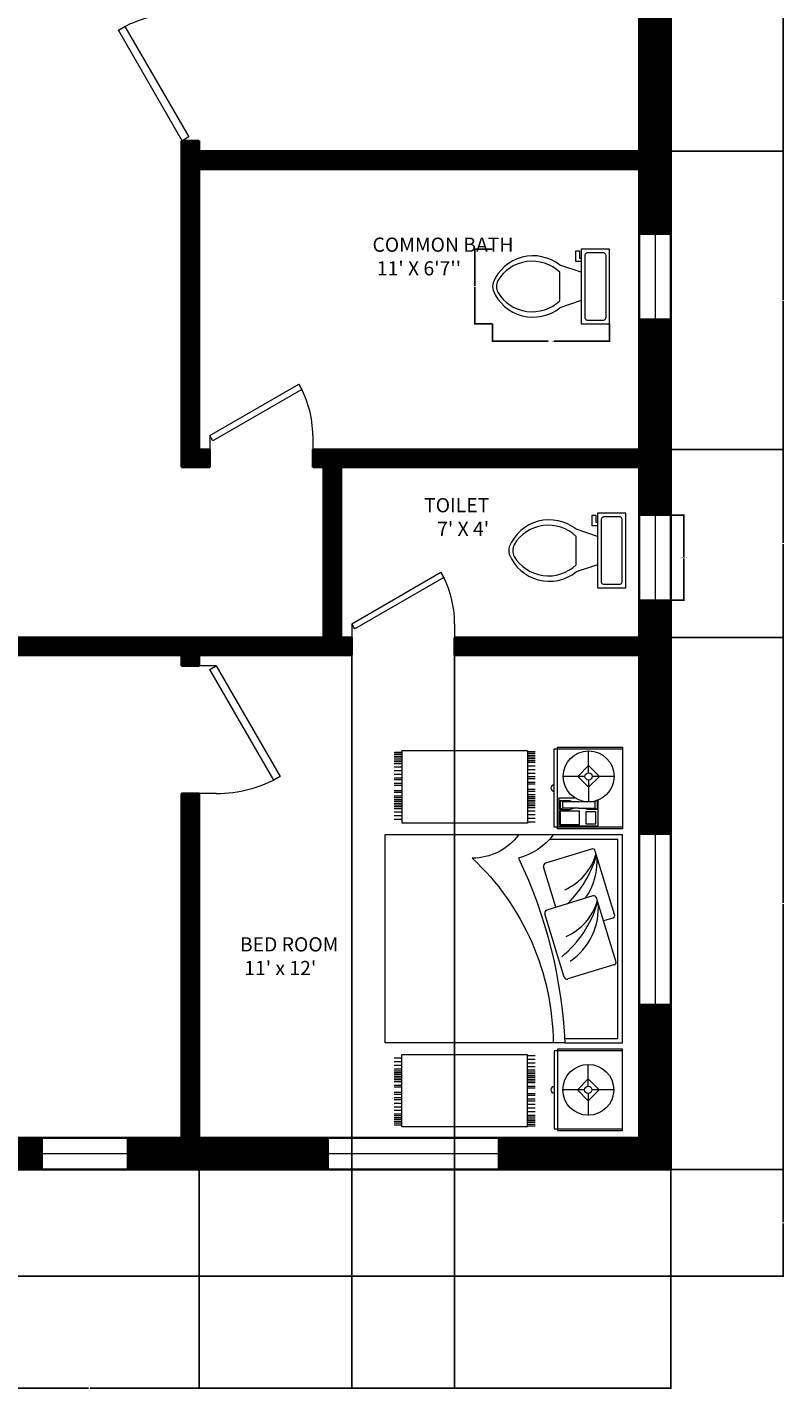
# Model space of a CAD drawing. Units: inches. Extents: x -19 to 404, y -21 to 673.
# Tile 2 of 3: x 191 to 404, y -21 to 363. Entities that reach past the tile are written whole.
import ezdxf

# ---------------------------------------------------------------- set-up
doc = ezdxf.new("R2010")
doc.units = ezdxf.units.IN
doc.header["$MEASUREMENT"] = 0
for name, color, linetype, lineweight in [('A-ANNO-DIMS', 2, 'Continuous', 18), ('A-AREA-IDEN', 7, 'Continuous', 18), ('A-WALL', 7, 'Continuous', 35), ('bathroom', 90, 'Continuous', 18), ('bedroom', 120, 'Continuous', 18), ('doors', 40, 'Continuous', 18), ('window', 30, 'Continuous', 18)]:
    doc.layers.add(name, color=color, linetype=linetype, lineweight=lineweight)
doc.layers.add('A-WALL-PATT', color=244, linetype='Continuous', lineweight=13, true_color=0x991b1e)
doc.styles.get("Standard").update_dxf_attribs({"font": 'arial.ttf'})
doc.dimstyles.get("Standard").update_dxf_attribs({"dimtxt": 0.18, "dimasz": 0.18, "dimexe": 0.18, "dimexo": 0.0625, "dimgap": 0.09, "dimtad": 0, "dimtih": 1, "dimtoh": 1, "dimdec": 4, "dimzin": 0, "dimdsep": 46, "dimtxsty": 'Standard', "dimcen": 0.09, "dimadec": 0, "dimazin": 0, "dimtfac": 1, "dimtdec": 4, "dimtofl": 0, "dimtmove": 0, "dimatfit": 3, "dimfxl": 1, "dimtolj": 1, "dimtzin": 0, "dimarcsym": 0})

# ---------------------------------------------------------------- blocks, each defined once
blk = doc.blocks.new('*U5')
for p, q in [((0, 0), (0, -100)), ((750, 0), (750, -100))]:
    blk.add_line(p, q)
blk.add_lwpolyline([(0, 0), (649.5, 375), (671.4, 337.1), (21.9, -37.9)], close=True)
blk.add_arc((0, 0), 750, 0, 30)
blk = doc.blocks.new('3')
for p, q in [((185.866, 224.677), (185.866, 225.236)), ((185.866, 225.236), (186.566, 225.236)), ((185.88, 224.649), (185.88, 225.236)), ((186.552, 225.236), (186.552, 224.649)), ((186.566, 225.236), (186.566, 224.677)), ((186.62, 225.236), (186.62, 224.64)), ((188.409, 225.236), (186.62, 225.236)), ((188.409, 224.739), (188.409, 225.236)), ((188.463, 225.236), (188.463, 224.677)), ((189.162, 225.236), (188.463, 225.236)), ((188.477, 225.236), (188.477, 224.649)), ((189.148, 224.649), (189.148, 225.236)), ((189.162, 224.677), (189.162, 225.236)), ((186.116, 225.164), (186.116, 224.976)), ((187.303, 225.168), (186.758, 225.001)), ((187.706, 225.179), (187.161, 225.012)), ((187.334, 225.152), (187.359, 225.073)), ((187.737, 225.163), (187.858, 224.766)), ((188.812, 225.162), (188.812, 224.974)), ((186.022, 224.945), (186.116, 225.039)), ((186.116, 225.039), (186.21, 224.945)), ((186.54, 225.027), (186.319, 225.027)), ((186.321, 225.017), (186.401, 225.017)), ((186.333, 224.997), (186.321, 225.017)), ((186.334, 224.858), (186.333, 224.997)), ((186.333, 224.997), (186.389, 224.997)), ((186.401, 225.017), (186.389, 224.997)), ((186.39, 224.858), (186.389, 224.997)), ((186.401, 225.017), (186.401, 224.938)), ((186.541, 224.69), (186.54, 225.027)), ((186.742, 224.97), (186.863, 224.573)), ((187.144, 224.981), (187.266, 224.584)), ((188.812, 225.036), (188.718, 224.942)), ((188.907, 224.942), (188.812, 225.036)), ((186.084, 224.945), (185.896, 224.945)), ((186.116, 224.851), (186.022, 224.945)), ((186.21, 224.945), (186.116, 224.851)), ((186.116, 224.914), (186.116, 224.726)), ((186.147, 224.945), (186.335, 224.945)), ((186.331, 224.905), (186.334, 224.898)), ((186.334, 224.858), (186.334, 224.719)), ((186.401, 224.938), (186.389, 224.898)), ((186.39, 224.858), (186.39, 224.719)), ((188.781, 224.942), (188.593, 224.942)), ((188.718, 224.942), (188.812, 224.848)), ((188.812, 224.848), (188.907, 224.942)), ((188.812, 224.911), (188.812, 224.723)), ((188.844, 224.942), (189.032, 224.942)), ((186.302, 224.83), (186.303, 224.689)), ((186.322, 224.779), (186.334, 224.818)), ((186.323, 224.699), (186.322, 224.779)), ((186.402, 224.779), (186.39, 224.819)), ((186.402, 224.7), (186.402, 224.779)), ((187.842, 224.735), (187.297, 224.568)), ((188.409, 224.739), (188.409, 223.191)), ((186.566, 224.677), (185.866, 224.677)), ((186.552, 224.649), (185.88, 224.649)), ((186.303, 224.689), (186.541, 224.69)), ((186.334, 224.719), (186.323, 224.699)), ((186.323, 224.699), (186.402, 224.7)), ((186.334, 224.719), (186.39, 224.719)), ((186.402, 224.7), (186.39, 224.719)), ((186.62, 224.64), (186.62, 223.191)), ((187.242, 224.663), (186.894, 224.557)), ((188.463, 224.677), (189.162, 224.677)), ((188.477, 224.649), (189.148, 224.649)), ((185.897, 224.42, -0.909), (185.897, 223.338, -0.909)), ((185.897, 224.42, -0.909), (186.517, 224.42, -0.909)), ((185.904, 224.485, -0.909), (185.904, 224.42, -0.909)), ((185.92, 224.485, -0.909), (185.92, 224.42, -0.909)), ((185.92, 224.485, -0.909), (185.92, 224.42, -0.909)), ((185.935, 224.485, -0.909), (185.935, 224.42, -0.909)), ((185.951, 224.485, -0.909), (185.951, 224.42, -0.909)), ((185.966, 224.485, -0.909), (185.966, 224.42, -0.909)), ((185.982, 224.485, -0.909), (185.982, 224.42, -0.909)), ((185.997, 224.485, -0.909), (185.997, 224.42, -0.909)), ((186.028, 224.485, -0.909), (186.028, 224.42, -0.909)), ((186.059, 224.485, -0.909), (186.059, 224.42, -0.909)), ((186.09, 224.485, -0.909), (186.09, 224.42, -0.909)), ((186.09, 224.485, -0.909), (186.09, 224.42, -0.909)), ((186.121, 224.485, -0.909), (186.121, 224.42, -0.909)), ((186.137, 224.485, -0.909), (186.137, 224.42, -0.909)), ((186.168, 224.485, -0.909), (186.168, 224.42, -0.909)), ((186.183, 224.485, -0.909), (186.183, 224.42, -0.909)), ((186.23, 224.485, -0.909), (186.23, 224.42, -0.909)), ((186.245, 224.485, -0.909), (186.245, 224.42, -0.909)), ((186.276, 224.485, -0.909), (186.276, 224.42, -0.909)), ((186.292, 224.485, -0.909), (186.292, 224.42, -0.909)), ((186.307, 224.485, -0.909), (186.307, 224.42, -0.909)), ((186.323, 224.485, -0.909), (186.323, 224.42, -0.909)), ((186.338, 224.485, -0.909), (186.338, 224.42, -0.909)), ((186.354, 224.485, -0.909), (186.354, 224.42, -0.909)), ((186.369, 224.485, -0.909), (186.369, 224.42, -0.909)), ((186.385, 224.485, -0.909), (186.385, 224.42, -0.909)), ((186.416, 224.485, -0.909), (186.416, 224.42, -0.909)), ((186.447, 224.485, -0.909), (186.447, 224.42, -0.909)), ((186.478, 224.485, -0.909), (186.478, 224.42, -0.909)), ((186.509, 224.485, -0.909), (186.509, 224.42, -0.909)), ((186.517, 224.42, -0.909), (186.517, 223.338, -0.909)), ((189.131, 224.42, -0.909), (188.511, 224.42, -0.909)), ((188.511, 224.42, -0.909), (188.511, 223.338, -0.909)), ((188.52, 224.485, -0.909), (188.52, 224.42, -0.909)), ((188.551, 224.485, -0.909), (188.551, 224.42, -0.909)), ((188.582, 224.485, -0.909), (188.582, 224.42, -0.909)), ((188.613, 224.485, -0.909), (188.613, 224.42, -0.909)), ((188.644, 224.485, -0.909), (188.644, 224.42, -0.909)), ((188.66, 224.485, -0.909), (188.66, 224.42, -0.909)), ((188.675, 224.485, -0.909), (188.675, 224.42, -0.909)), ((188.691, 224.485, -0.909), (188.691, 224.42, -0.909)), ((188.706, 224.485, -0.909), (188.706, 224.42, -0.909)), ((188.722, 224.485, -0.909), (188.722, 224.42, -0.909)), ((188.737, 224.485, -0.909), (188.737, 224.42, -0.909)), ((188.753, 224.485, -0.909), (188.753, 224.42, -0.909)), ((188.784, 224.485, -0.909), (188.784, 224.42, -0.909)), ((188.799, 224.485, -0.909), (188.799, 224.42, -0.909)), ((188.846, 224.485, -0.909), (188.846, 224.42, -0.909)), ((188.861, 224.485, -0.909), (188.861, 224.42, -0.909)), ((188.892, 224.485, -0.909), (188.892, 224.42, -0.909)), ((188.908, 224.485, -0.909), (188.908, 224.42, -0.909)), ((188.939, 224.485, -0.909), (188.939, 224.42, -0.909)), ((188.939, 224.485, -0.909), (188.939, 224.42, -0.909)), ((188.97, 224.485, -0.909), (188.97, 224.42, -0.909)), ((189.001, 224.485, -0.909), (189.001, 224.42, -0.909)), ((189.032, 224.485, -0.909), (189.032, 224.42, -0.909)), ((189.047, 224.485, -0.909), (189.047, 224.42, -0.909)), ((189.063, 224.485, -0.909), (189.063, 224.42, -0.909)), ((189.078, 224.485, -0.909), (189.078, 224.42, -0.909)), ((189.094, 224.485, -0.909), (189.094, 224.42, -0.909)), ((189.109, 224.485, -0.909), (189.109, 224.42, -0.909)), ((189.109, 224.485, -0.909), (189.109, 224.42, -0.909)), ((189.125, 224.485, -0.909), (189.125, 224.42, -0.909)), ((189.131, 224.42, -0.909), (189.131, 223.338, -0.909)), ((185.897, 223.338, -0.909), (186.517, 223.338, -0.909)), ((185.911, 223.338, -0.909), (185.911, 223.279, -0.909)), ((185.911, 223.338, -0.909), (185.911, 223.279, -0.909)), ((185.911, 223.338, -0.909), (185.911, 223.279, -0.909)), ((185.914, 223.338, -0.909), (185.914, 223.273, -0.909)), ((185.929, 223.338, -0.909), (185.929, 223.273, -0.909)), ((185.929, 223.338, -0.909), (185.929, 223.273, -0.909)), ((185.945, 223.338, -0.909), (185.945, 223.273, -0.909)), ((185.96, 223.338, -0.909), (185.96, 223.273, -0.909)), ((185.976, 223.338, -0.909), (185.976, 223.273, -0.909)), ((185.991, 223.338, -0.909), (185.991, 223.273, -0.909)), ((186.007, 223.338, -0.909), (186.007, 223.273, -0.909)), ((186.038, 223.338, -0.909), (186.038, 223.273, -0.909)), ((186.069, 223.338, -0.909), (186.069, 223.273, -0.909)), ((186.1, 223.338, -0.909), (186.1, 223.273, -0.909)), ((186.1, 223.338, -0.909), (186.1, 223.273, -0.909)), ((186.131, 223.338, -0.909), (186.131, 223.273, -0.909)), ((186.146, 223.338, -0.909), (186.146, 223.273, -0.909)), ((186.177, 223.338, -0.909), (186.177, 223.273, -0.909)), ((186.193, 223.338, -0.909), (186.193, 223.273, -0.909)), ((186.239, 223.338, -0.909), (186.239, 223.273, -0.909)), ((186.255, 223.338, -0.909), (186.255, 223.273, -0.909)), ((186.286, 223.338, -0.909), (186.286, 223.273, -0.909)), ((186.301, 223.338, -0.909), (186.301, 223.273, -0.909)), ((186.317, 223.338, -0.909), (186.317, 223.273, -0.909)), ((186.332, 223.338, -0.909), (186.332, 223.273, -0.909)), ((186.348, 223.338, -0.909), (186.348, 223.273, -0.909)), ((186.363, 223.338, -0.909), (186.363, 223.273, -0.909)), ((186.379, 223.338, -0.909), (186.379, 223.273, -0.909)), ((186.394, 223.338, -0.909), (186.394, 223.273, -0.909)), ((186.425, 223.338, -0.909), (186.425, 223.273, -0.909)), ((186.456, 223.338, -0.909), (186.456, 223.273, -0.909)), ((186.487, 223.338, -0.909), (186.487, 223.273, -0.909)), ((189.131, 223.338, -0.909), (188.511, 223.338, -0.909)), ((188.541, 223.338, -0.909), (188.541, 223.273, -0.909)), ((188.572, 223.338, -0.909), (188.572, 223.273, -0.909)), ((188.603, 223.338, -0.909), (188.603, 223.273, -0.909)), ((188.634, 223.338, -0.909), (188.634, 223.273, -0.909)), ((188.65, 223.338, -0.909), (188.65, 223.273, -0.909)), ((188.665, 223.338, -0.909), (188.665, 223.273, -0.909)), ((188.681, 223.338, -0.909), (188.681, 223.273, -0.909)), ((188.696, 223.338, -0.909), (188.696, 223.273, -0.909)), ((188.712, 223.338, -0.909), (188.712, 223.273, -0.909)), ((188.727, 223.338, -0.909), (188.727, 223.273, -0.909)), ((188.743, 223.338, -0.909), (188.743, 223.273, -0.909)), ((188.774, 223.338, -0.909), (188.774, 223.273, -0.909)), ((188.789, 223.338, -0.909), (188.789, 223.273, -0.909)), ((188.836, 223.338, -0.909), (188.836, 223.273, -0.909)), ((188.851, 223.338, -0.909), (188.851, 223.273, -0.909)), ((188.882, 223.338, -0.909), (188.882, 223.273, -0.909)), ((188.898, 223.338, -0.909), (188.898, 223.273, -0.909)), ((188.929, 223.338, -0.909), (188.929, 223.273, -0.909)), ((188.929, 223.338, -0.909), (188.929, 223.273, -0.909)), ((188.96, 223.338, -0.909), (188.96, 223.273, -0.909)), ((188.991, 223.338, -0.909), (188.991, 223.273, -0.909)), ((189.022, 223.338, -0.909), (189.022, 223.273, -0.909)), ((189.037, 223.338, -0.909), (189.037, 223.273, -0.909)), ((189.053, 223.338, -0.909), (189.053, 223.273, -0.909)), ((189.068, 223.338, -0.909), (189.068, 223.273, -0.909)), ((189.084, 223.338, -0.909), (189.084, 223.273, -0.909)), ((189.099, 223.338, -0.909), (189.099, 223.273, -0.909)), ((189.099, 223.338, -0.909), (189.099, 223.273, -0.909)), ((189.115, 223.338, -0.909), (189.115, 223.273, -0.909)), ((189.117, 223.338, -0.909), (189.117, 223.279, -0.909)), ((189.117, 223.338, -0.909), (189.117, 223.279, -0.909)), ((189.117, 223.338, -0.909), (189.117, 223.279, -0.909)), ((186.62, 223.191), (188.409, 223.191))]:
    blk.add_line(p, q)
blk.add_lwpolyline([(188.369, 224.737), (188.369, 225.197), (186.66, 225.197), (186.66, 224.606)])
for points in [[(186.422, 225.007), (186.422, 224.92), (186.525, 224.92), (186.525, 225.008)], [(186.415, 224.866), (186.416, 224.7), (186.531, 224.7), (186.53, 224.867)]]:
    blk.add_lwpolyline(points, close=True)
for points in [[(186.62, 224.64, -0.162278), (186.819, 224.342, -0.100664), (188.409, 224.739, -0.100664)], [(186.62, 224.342, -0.236068), (186.819, 223.944, -0.205258), (188.409, 224.64, -0.205258)]]:
    blk.add_lwpolyline(points, format="xyb")
for centre, radius in [((186.116, 224.945), 0.219), ((188.812, 224.942), 0.219), ((186.116, 224.945), 0.0313), ((188.812, 224.942), 0.0313)]:
    blk.add_circle(centre, radius)
for centre, radius, start, end in [((187.311, 225.145), 0.0248, 17.0142, 107.0142), ((187.713, 225.156), 0.0248, 17.0142, 107.0142), ((186.765, 224.978), 0.0248, 107.0142, 197.0142), ((186.647, 224.541), 0.487, 24.2209, 73.0691), ((186.848, 224.471), 0.547, 54.6851, 95.1605), ((186.536, 224.105), 0.943, 44.2727, 73.7189), ((187.168, 224.989), 0.0248, 107.0142, 197.0142), ((187.05, 224.552), 0.487, 24.2209, 73.0691), ((187.25, 224.482), 0.547, 33.7801, 95.1605), ((186.938, 224.116), 0.943, 39.4023, 73.7189), ((187.835, 224.758), 0.0248, 287.0142, 17.0142), ((186.216, 224.649), 0.028, 180, 0), ((188.812, 224.649), 0.028, 180, 0), ((186.887, 224.581), 0.0248, 197.0142, 287.0142), ((187.289, 224.592), 0.0248, 197.0142, 287.0142)]:
    blk.add_arc(centre, radius, start, end)
blk = doc.blocks.new('Toilet - top')
for p, q in [((9.5, -6), (9.5, -2)), ((-10, -8.5), (-8, -8.5)), ((-10, -9.5), (-10, -8.5)), ((-7, -9.5), (-10, -9.5)), ((-8, -8.5), (-8, -8)), ((-7, -8), (-7, -9.5)), ((-4, -8), (-6, -14)), ((4, -8), (6, -14)), ((4, -14), (-4, -14))]:
    blk.add_line(p, q)
blk.add_lwpolyline([(10.5, -8), (10.5, 0), (-10.5, 0), (-10.5, -8)], close=True)
for points in [[(-9.5, -2), (-9.5, -6)], [(8.5, -1), (-8.5, -1)], [(-8.5, -7), (8.5, -7)]]:
    blk.add_lwpolyline(points)
for centre, radius, start, end in [((-8.62, -1.88), 0.884, 81.8699, 188.1301), ((8.62, -1.88), 0.884, 351.8699, 98.1301), ((-8.62, -6.12), 0.884, 171.8699, 278.1301), ((8.62, -6.12), 0.884, 261.8699, 8.1301), ((3.52, -21.58), 12.17, 141.4691, 247.9714), ((4.2, -21.82), 11.33, 136.3677, 238.9468), ((-3.52, -21.58), 12.17, 292.0284, 38.5307), ((-4.2, -21.82), 11.33, 301.053, 43.6321), ((0, -27.88), 4, 245.7318, 294.2682), ((0, -29), 4, 254.8605, 285.1395)]:
    blk.add_arc(centre, radius, start, end)
blk = doc.blocks.new('WIN-48IN')
for p, q in [((0, 48), (9, 48)), ((0, 0), (0, 48)), ((0, 48), (4.5, 48)), ((4.5, 48), (4.5, 0)), ((9, 48), (9, 0)), ((9, 0), (0, 0))]:
    blk.add_line(p, q)
blk = doc.blocks.new('WIN-24IN')
for p, q in [((0, 24), (9, 24)), ((0, 0), (0, 24)), ((0, 24), (4.5, 24)), ((4.5, 24), (4.5, 0)), ((9, 24), (9, 0)), ((9, 0), (0, 0))]:
    blk.add_line(p, q)
blk = doc.blocks.new('*D15')
at = {"layer": 'A-ANNO-DIMS', "color": 0, "lineweight": -2, "transparency": 16777216}
for p, q in [((372.71, 225.27), (376.43, 225.27)), ((376.25, 225.09), (376.25, 213.45)), ((376.25, 201.45), (376.25, 213.09)), ((372.71, 201.27), (376.43, 201.27))]:
    blk.add_line(p, q, dxfattribs=at)
at = {"layer": 'A-ANNO-DIMS', "color": 0, "transparency": 16777216}
for points in [[(376.22, 225.09), (376.28, 225.09), (376.25, 225.27)], [(376.22, 201.45), (376.28, 201.45), (376.25, 201.27)]]:
    blk.add_solid(points, dxfattribs=at)
at = {"layer": 'Defpoints', "color": 0, "transparency": 16777216}
for p in [(372.65, 225.27), (376.25, 225.27), (372.65, 201.27)]:
    blk.add_point(p, dxfattribs=at)
at = {"layer": 'A-ANNO-DIMS', "color": 0, "transparency": 16777216, "insert": (376.25, 213.27), "char_height": 0.18, "attachment_point": 5}
blk.add_mtext('\\A1;WINDOW 24 TYP.', dxfattribs=at)
blk = doc.blocks.new('*D16')
at = {"layer": 'A-ANNO-DIMS', "color": 0, "lineweight": -2, "transparency": 16777216}
for p, q in [((363.65, 201.21), (363.65, 197.49)), ((372.65, 201.21), (372.65, 197.49)), ((363.83, 197.67), (367.69, 197.67)), ((372.47, 197.67), (368.61, 197.67))]:
    blk.add_line(p, q, dxfattribs=at)
at = {"layer": 'A-ANNO-DIMS', "color": 0, "transparency": 16777216}
for points in [[(363.83, 197.7), (363.83, 197.64), (363.65, 197.67)], [(372.47, 197.7), (372.47, 197.64), (372.65, 197.67)]]:
    blk.add_solid(points, dxfattribs=at)
at = {"layer": 'Defpoints', "color": 0, "transparency": 16777216}
for p in [(363.65, 201.27), (372.65, 201.27), (372.65, 197.67)]:
    blk.add_point(p, dxfattribs=at)
at = {"layer": 'A-ANNO-DIMS', "color": 0, "transparency": 16777216, "insert": (368.15, 197.67), "char_height": 0.18, "attachment_point": 5}
blk.add_mtext('\\A1;9 TYP.', dxfattribs=at)
blk = doc.blocks.new('*D17')
at = {"layer": 'A-ANNO-DIMS', "color": 0, "lineweight": -2, "transparency": 16777216}
for p, q in [((322.29, 279.16), (322.29, 274.09)), ((355.34, 279.16), (355.34, 274.09)), ((322.47, 274.27), (338.04, 274.27)), ((355.16, 274.27), (339.59, 274.27))]:
    blk.add_line(p, q, dxfattribs=at)
at = {"layer": 'A-ANNO-DIMS', "color": 0, "transparency": 16777216}
for points in [[(322.47, 274.3), (322.47, 274.24), (322.29, 274.27)], [(355.16, 274.3), (355.16, 274.24), (355.34, 274.27)]]:
    blk.add_solid(points, dxfattribs=at)
at = {"layer": 'Defpoints', "color": 0, "transparency": 16777216}
for p in [(322.29, 279.23), (355.34, 279.23), (355.34, 274.27)]:
    blk.add_point(p, dxfattribs=at)
at = {"layer": 'A-ANNO-DIMS', "color": 0, "transparency": 16777216, "insert": (338.81, 274.27), "char_height": 0.18, "attachment_point": 5}
blk.add_mtext('\\A1;WC 33 TYP.', dxfattribs=at)
blk = doc.blocks.new('*D18')
at = {"layer": 'A-ANNO-DIMS', "color": 0, "lineweight": -2, "transparency": 16777216}
for p, q in [((322.23, 300.23), (317.15, 300.23)), ((317.33, 300.05), (317.33, 289.91)), ((317.33, 279.41), (317.33, 289.55)), ((322.23, 279.23), (317.15, 279.23))]:
    blk.add_line(p, q, dxfattribs=at)
at = {"layer": 'A-ANNO-DIMS', "color": 0, "transparency": 16777216}
for points in [[(317.3, 300.05), (317.36, 300.05), (317.33, 300.23)], [(317.3, 279.41), (317.36, 279.41), (317.33, 279.23)]]:
    blk.add_solid(points, dxfattribs=at)
at = {"layer": 'Defpoints', "color": 0, "transparency": 16777216}
for p in [(322.29, 300.23), (317.33, 279.23), (322.29, 279.23)]:
    blk.add_point(p, dxfattribs=at)
at = {"layer": 'A-ANNO-DIMS', "color": 0, "transparency": 16777216, "insert": (317.33, 289.73), "char_height": 0.18, "attachment_point": 5}
blk.add_mtext('\\A1;21 TYP.', dxfattribs=at)
blk = doc.blocks.new('*D27')
at = {"layer": 'A-ANNO-DIMS', "color": 0, "lineweight": -2, "transparency": 16777216}
for p, q in [((372.71, 40.82), (404.42, 40.82)), ((404.24, 40.64), (404.24, 26)), ((404.24, 11), (404.24, 25.64)), ((177.71, 10.82), (404.42, 10.82))]:
    blk.add_line(p, q, dxfattribs=at)
at = {"layer": 'A-ANNO-DIMS', "color": 0, "transparency": 16777216}
for points in [[(404.21, 40.64), (404.27, 40.64), (404.24, 40.82)], [(404.21, 11), (404.27, 11), (404.24, 10.82)]]:
    blk.add_solid(points, dxfattribs=at)
at = {"layer": 'Defpoints', "color": 0, "transparency": 16777216}
for p in [(372.65, 40.82), (177.65, 10.82), (404.24, 10.82)]:
    blk.add_point(p, dxfattribs=at)
at = {"layer": 'A-ANNO-DIMS', "color": 0, "transparency": 16777216, "insert": (404.24, 25.82), "char_height": 0.18, "attachment_point": 5}
blk.add_mtext('\\A1;30', dxfattribs=at)
blk = doc.blocks.new('*D30')
at = {"layer": 'A-ANNO-DIMS', "color": 0, "lineweight": -2, "transparency": 16777216}
for p, q in [((239.65, 49.76), (239.65, -20.95)), ((177.65, 10.76), (177.65, -20.95)), ((177.83, -20.77), (208.43, -20.77)), ((239.47, -20.77), (208.87, -20.77))]:
    blk.add_line(p, q, dxfattribs=at)
at = {"layer": 'A-ANNO-DIMS', "color": 0, "transparency": 16777216}
for points in [[(177.83, -20.74), (177.83, -20.8), (177.65, -20.77)], [(239.47, -20.74), (239.47, -20.8), (239.65, -20.77)]]:
    blk.add_solid(points, dxfattribs=at)
at = {"layer": 'Defpoints', "color": 0, "transparency": 16777216}
for p in [(239.65, 49.82), (177.65, 10.82), (239.65, -20.77)]:
    blk.add_point(p, dxfattribs=at)
at = {"layer": 'A-ANNO-DIMS', "color": 0, "transparency": 16777216, "insert": (208.65, -20.77), "char_height": 0.18, "attachment_point": 5}
blk.add_mtext('\\A1;62', dxfattribs=at)
blk = doc.blocks.new('*D31')
at = {"layer": 'A-ANNO-DIMS', "color": 0, "lineweight": -2, "transparency": 16777216}
for p, q in [((239.65, 49.76), (239.65, -20.95)), ((372.65, 40.76), (372.65, -20.95)), ((239.83, -20.77), (305.87, -20.77)), ((372.47, -20.77), (306.43, -20.77))]:
    blk.add_line(p, q, dxfattribs=at)
at = {"layer": 'A-ANNO-DIMS', "color": 0, "transparency": 16777216}
for points in [[(239.83, -20.74), (239.83, -20.8), (239.65, -20.77)], [(372.47, -20.74), (372.47, -20.8), (372.65, -20.77)]]:
    blk.add_solid(points, dxfattribs=at)
at = {"layer": 'Defpoints', "color": 0, "transparency": 16777216}
for p in [(239.65, 49.82), (372.65, 40.82), (372.65, -20.77)]:
    blk.add_point(p, dxfattribs=at)
at = {"layer": 'A-ANNO-DIMS', "color": 0, "transparency": 16777216, "insert": (306.15, -20.77), "char_height": 0.18, "attachment_point": 5}
blk.add_mtext('\\A1;133', dxfattribs=at)
blk = doc.blocks.new('*D33')
at = {"layer": 'A-ANNO-DIMS', "color": 0, "lineweight": -2, "transparency": 16777216}
for p, q in [((363.71, 487.82), (404.42, 487.82)), ((404.24, 487.64), (404.24, 408)), ((404.24, 328), (404.24, 407.64)), ((363.71, 327.82), (404.42, 327.82))]:
    blk.add_line(p, q, dxfattribs=at)
at = {"layer": 'A-ANNO-DIMS', "color": 0, "transparency": 16777216}
for points in [[(404.21, 487.64), (404.27, 487.64), (404.24, 487.82)], [(404.21, 328), (404.27, 328), (404.24, 327.82)]]:
    blk.add_solid(points, dxfattribs=at)
at = {"layer": 'Defpoints', "color": 0, "transparency": 16777216}
for p in [(363.65, 487.82), (404.24, 487.82), (363.65, 327.82)]:
    blk.add_point(p, dxfattribs=at)
at = {"layer": 'A-ANNO-DIMS', "color": 0, "transparency": 16777216, "insert": (404.24, 407.82), "char_height": 0.18, "attachment_point": 5}
blk.add_mtext('\\A1;160', dxfattribs=at)
blk = doc.blocks.new('*D34')
at = {"layer": 'A-ANNO-DIMS', "color": 0, "lineweight": -2, "transparency": 16777216}
for p, q in [((363.71, 327.82), (404.42, 327.82)), ((404.24, 327.64), (404.24, 286)), ((404.24, 244), (404.24, 285.64)), ((363.71, 243.82), (404.42, 243.82))]:
    blk.add_line(p, q, dxfattribs=at)
at = {"layer": 'A-ANNO-DIMS', "color": 0, "transparency": 16777216}
for points in [[(404.21, 327.64), (404.27, 327.64), (404.24, 327.82)], [(404.21, 244), (404.27, 244), (404.24, 243.82)]]:
    blk.add_solid(points, dxfattribs=at)
at = {"layer": 'Defpoints', "color": 0, "transparency": 16777216}
for p in [(363.65, 327.82), (404.24, 327.82), (363.65, 243.82)]:
    blk.add_point(p, dxfattribs=at)
at = {"layer": 'A-ANNO-DIMS', "color": 0, "transparency": 16777216, "insert": (404.24, 285.82), "char_height": 0.18, "attachment_point": 5}
blk.add_mtext('\\A1;84', dxfattribs=at)
blk = doc.blocks.new('*D35')
at = {"layer": 'A-ANNO-DIMS', "color": 0, "lineweight": -2, "transparency": 16777216}
for p, q in [((363.71, 243.82), (404.42, 243.82)), ((404.24, 243.64), (404.24, 217.5)), ((404.24, 191), (404.24, 217.14)), ((363.71, 190.82), (404.42, 190.82))]:
    blk.add_line(p, q, dxfattribs=at)
at = {"layer": 'A-ANNO-DIMS', "color": 0, "transparency": 16777216}
for points in [[(404.21, 243.64), (404.27, 243.64), (404.24, 243.82)], [(404.21, 191), (404.27, 191), (404.24, 190.82)]]:
    blk.add_solid(points, dxfattribs=at)
at = {"layer": 'Defpoints', "color": 0, "transparency": 16777216}
for p in [(363.65, 243.82), (404.24, 243.82), (363.65, 190.82)]:
    blk.add_point(p, dxfattribs=at)
at = {"layer": 'A-ANNO-DIMS', "color": 0, "transparency": 16777216, "insert": (404.24, 217.32), "char_height": 0.18, "attachment_point": 5}
blk.add_mtext('\\A1;53', dxfattribs=at)
blk = doc.blocks.new('*D36')
at = {"layer": 'A-ANNO-DIMS', "color": 0, "lineweight": -2, "transparency": 16777216}
for p, q in [((363.71, 190.82), (404.42, 190.82)), ((404.24, 190.64), (404.24, 116)), ((404.24, 41), (404.24, 115.64)), ((372.71, 40.82), (404.42, 40.82))]:
    blk.add_line(p, q, dxfattribs=at)
at = {"layer": 'A-ANNO-DIMS', "color": 0, "transparency": 16777216}
for points in [[(404.21, 190.64), (404.27, 190.64), (404.24, 190.82)], [(404.21, 41), (404.27, 41), (404.24, 40.82)]]:
    blk.add_solid(points, dxfattribs=at)
at = {"layer": 'Defpoints', "color": 0, "transparency": 16777216}
for p in [(363.65, 190.82), (404.24, 190.82), (372.65, 40.82)]:
    blk.add_point(p, dxfattribs=at)
at = {"layer": 'A-ANNO-DIMS', "color": 0, "transparency": 16777216, "insert": (404.24, 115.82), "char_height": 0.18, "attachment_point": 5}
blk.add_mtext('\\A1;150', dxfattribs=at)
blk = doc.blocks.new('*D37')
at = {"layer": 'A-ANNO-DIMS', "color": 0, "lineweight": -2, "transparency": 16777216}
for p, q in [((282.65, 185.76), (282.65, -20.95)), ((311.65, 185.76), (311.65, -20.95)), ((282.83, -20.77), (296.93, -20.77)), ((311.47, -20.77), (297.37, -20.77))]:
    blk.add_line(p, q, dxfattribs=at)
at = {"layer": 'A-ANNO-DIMS', "color": 0, "transparency": 16777216}
for points in [[(282.83, -20.74), (282.83, -20.8), (282.65, -20.77)], [(311.47, -20.74), (311.47, -20.8), (311.65, -20.77)]]:
    blk.add_solid(points, dxfattribs=at)
at = {"layer": 'Defpoints', "color": 0, "transparency": 16777216}
for p in [(282.65, 185.82), (311.65, 185.82), (311.65, -20.77)]:
    blk.add_point(p, dxfattribs=at)
at = {"layer": 'A-ANNO-DIMS', "color": 0, "transparency": 16777216, "insert": (297.15, -20.77), "char_height": 0.18, "attachment_point": 5}
blk.add_mtext('\\A1;29', dxfattribs=at)

msp = doc.modelspace()

# ---------------------------------------------------------------- hatches: boundary and pattern name
at = {"layer": 'A-WALL-PATT'}
h = msp.add_hatch(dxfattribs=at)
h.set_pattern_fill('ANSI31', color=256)
h.set_pattern_definition([(45, (-13642.13922, -42713.83606), (-0.08838834765, 0.08838834765), [])])
h.paths.add_polyline_path([(195.39, 49.82), (177.65, 49.82), (177.65, 40.82), (195.39, 40.82)])
h.paths.add_polyline_path([(276.02, 49.82), (239.65, 49.82), (239.65, 146.82), (234.65, 146.82), (234.65, 49.82), (219.39, 49.82), (219.39, 40.82), (276.02, 40.82)])
h.paths.add_polyline_path([(372.65, 87.37), (363.65, 87.37), (363.65, 49.82), (324.02, 49.82), (324.02, 40.82), (372.65, 40.82)])
h.paths.add_polyline_path([(372.65, 280.5), (363.65, 280.5), (363.65, 243.82), (271.65, 243.82), (271.65, 238.82), (274.65, 238.82), (274.65, 190.82), (161.65, 190.82), (161.65, 185.82), (234.65, 185.82), (234.65, 182.82), (239.65, 182.82), (239.65, 185.82), (282.65, 185.82), (282.65, 190.82), (279.65, 190.82), (279.65, 238.82), (363.65, 238.82), (363.65, 225.27), (368.15, 225.27), (372.65, 225.27)])
h.paths.add_polyline_path([(372.65, 201.27), (363.65, 201.27), (363.65, 190.82), (311.65, 190.82), (311.65, 185.82), (363.65, 185.82), (363.65, 135.37), (368.15, 135.37), (372.65, 135.37)])
h.paths.add_polyline_path([(372.65, 383.98), (363.65, 383.98), (363.65, 327.82), (239.65, 327.82), (239.65, 330.82), (234.65, 330.82), (234.65, 327.82), (234.65, 238.82), (242.65, 238.82), (242.65, 243.82), (239.65, 243.82), (239.65, 322.82), (363.65, 322.82), (363.65, 304.5), (368.15, 304.5), (372.65, 304.5)])

# ---------------------------------------------------------------- linework, layer by layer
at = {"layer": 'A-WALL'}
for p, q in [((363.65, 482.82), (363.65, 327.82)), ((234.65, 238.82), (234.65, 330.82)), ((234.65, 327.82), (234.65, 330.82)), ((234.65, 330.82), (239.65, 330.82)), ((239.65, 327.82), (239.65, 330.82)), ((239.65, 327.82), (363.65, 327.82)), ((239.65, 322.82), (363.65, 322.82)), ((239.65, 243.82), (239.65, 322.82)), ((363.65, 322.82), (363.65, 243.82)), ((239.65, 243.82), (242.65, 243.82)), ((239.65, 243.82), (242.65, 243.82)), ((242.65, 243.82), (242.65, 238.82)), ((271.65, 243.82), (363.65, 243.82)), ((271.65, 238.82), (271.65, 243.82)), ((234.65, 238.82), (242.65, 238.82)), ((271.65, 238.82), (274.65, 238.82)), ((271.65, 238.82), (274.65, 238.82)), ((274.65, 238.82), (274.65, 190.82)), ((279.65, 238.82), (363.65, 238.82)), ((279.65, 238.82), (279.65, 190.82)), ((363.65, 238.82), (363.65, 190.82)), ((161.65, 190.82), (274.65, 190.82)), ((279.65, 190.82), (282.65, 190.82)), ((279.65, 190.82), (282.65, 190.82)), ((282.65, 190.82), (282.65, 185.82)), ((311.65, 190.82), (363.65, 190.82)), ((311.65, 185.82), (311.65, 190.82)), ((161.65, 185.82), (234.65, 185.82)), ((234.65, 182.82), (234.65, 185.82)), ((234.65, 185.82), (234.65, 182.82)), ((239.65, 185.82), (282.65, 185.82)), ((239.65, 182.82), (239.65, 185.82)), ((311.65, 185.82), (363.65, 185.82)), ((363.65, 185.82), (363.65, 49.82)), ((234.65, 182.82), (239.65, 182.82)), ((234.65, 49.82), (234.65, 146.82)), ((239.65, 146.82), (234.65, 146.82)), ((239.65, 49.82), (239.65, 146.82)), ((234.65, 49.82), (177.65, 49.82)), ((363.65, 49.82), (239.65, 49.82))]:
    msp.add_line(p, q, dxfattribs=at)
msp.add_lwpolyline([(114.65, 40.82), (12.65, 40.82), (12.65, 640.82), (372.65, 640.82), (372.65, 40.82), (177.65, 40.82)], dxfattribs=at)

# ---------------------------------------------------------------- block references
at = {"layer": 'bathroom', "rotation": 270}
for p in [(355.34, 289.73), (359.92, 215.29)]:
    msp.add_blockref('Toilet - top', p, dxfattribs=at)
at = {"layer": 'bedroom', "xscale": 32.76894482774335, "yscale": 32.76894482774335, "zscale": 32.76894482774335, "rotation": 270}
msp.add_blockref('3', (-7021.78, 6250.47), dxfattribs=at)
at = {"layer": 'doors', "xscale": 0.0480000000000013, "yscale": 0.0480000000000013, "zscale": 0.0480000000000013}
for p, rotation in [((234.85, 330.82), 90), ((244.45, 182.82), 270)]:
    msp.add_blockref('*U5', p, dxfattribs=dict(at, rotation=rotation))
at = {"layer": 'doors', "xscale": 0.0386666666666677, "yscale": 0.0386666666666677, "zscale": 0.0386666666666677}
for p in [(242.65, 247.69), (282.65, 194.69)]:
    msp.add_blockref('*U5', p, dxfattribs=at)
at = {"layer": 'window'}
for name, p in [('WIN-24IN', (363.65, 280.5)), ('WIN-24IN', (363.65, 201.27)), ('WIN-48IN', (363.65, 87.37))]:
    msp.add_blockref(name, p, dxfattribs=at)
at = {"layer": 'window', "extrusion": (0, 0, -1), "zscale": -1}
for name, p, rotation in [('WIN-24IN', (-219.39, 49.82), 269.999999999999), ('WIN-48IN', (-324.02, 49.82), 270.0000000000001)]:
    msp.add_blockref(name, p, dxfattribs=dict(at, rotation=rotation))

# ---------------------------------------------------------------- texts
at = {"layer": 'A-AREA-IDEN', "char_height": 4, "attachment_point": 1}
for s, insert in [("   COMMON BATH\\P    11' X 6'7''", (284.82, 303.51)), ("  TOILET\\P     7' X 4'", (300.6, 230.08)), ("  BED ROOM\\P   11' x 12'", (248.67, 106.3))]:
    msp.add_mtext_dynamic_manual_height_columns(s, width=75.0771, gutter_width=1, heights=[0], dxfattribs=dict(at, insert=insert))

# ---------------------------------------------------------------- dimensions: what is measured, and where the dimension line sits
at = {"layer": 'A-ANNO-DIMS'}
for base, p1, p2, picture, middle in [((404.24, 487.82), (363.65, 327.82), (363.65, 487.82), '*D33', (404.24, 407.82)), ((404.24, 327.82), (363.65, 243.82), (363.65, 327.82), '*D34', (404.24, 285.82)), ((404.24, 243.82), (363.65, 190.82), (363.65, 243.82), '*D35', (404.24, 217.32)), ((404.24, 190.82), (372.65, 40.82), (363.65, 190.82), '*D36', (404.24, 115.82)), ((404.24, 10.82), (372.65, 40.82), (177.65, 10.82), '*D27', (404.24, 25.82))]:
    dim = msp.add_linear_dim(base=base, p1=p1, p2=p2, angle=90, dimstyle='Standard', override={"dimdec": 0, "dimlfac": 1, "dimrnd": 0, "dimzin": 0, "dimdsep": 46, "dimlunit": 2}, dxfattribs=at)
    dim.commit()
    dim.dimension.update_dxf_attribs({"geometry": picture, "text_midpoint": middle})
for base, p1, p2, angle, text, picture, middle in [((317.33, 279.23), (322.29, 300.23), (322.29, 279.23), 270, '<> TYP.', '*D18', (317.33, 289.73)), ((376.25, 225.27), (372.65, 201.27), (372.65, 225.27), 90, 'WINDOW <> TYP.', '*D15', (376.25, 213.27))]:
    dim = msp.add_linear_dim(base=base, p1=p1, p2=p2, angle=angle, text=text, dimstyle='Standard', override={"dimdec": 0, "dimlfac": 1, "dimrnd": 0, "dimzin": 0, "dimdsep": 46, "dimlunit": 2}, dxfattribs=at)
    dim.commit()
    dim.dimension.update_dxf_attribs({"geometry": picture, "text_midpoint": middle})
for base, p1, p2, text, picture, middle in [((355.34, 274.27), (322.29, 279.23), (355.34, 279.23), 'WC <> TYP.', '*D17', (338.81, 274.27)), ((372.65, 197.67), (363.65, 201.27), (372.65, 201.27), '<> TYP.', '*D16', (368.15, 197.67))]:
    dim = msp.add_linear_dim(base=base, p1=p1, p2=p2, text=text, dimstyle='Standard', override={"dimdec": 0, "dimlfac": 1, "dimrnd": 0, "dimzin": 0, "dimdsep": 46, "dimlunit": 2}, dxfattribs=at)
    dim.commit()
    dim.dimension.update_dxf_attribs({"geometry": picture, "text_midpoint": middle})
for base, p1, p2, picture, middle in [((311.65, -20.77), (282.65, 185.82), (311.65, 185.82), '*D37', (297.15, -20.77)), ((239.65, -20.77), (177.65, 10.82), (239.65, 49.82), '*D30', (208.65, -20.77)), ((372.65, -20.77), (239.65, 49.82), (372.65, 40.82), '*D31', (306.15, -20.77))]:
    dim = msp.add_linear_dim(base=base, p1=p1, p2=p2, dimstyle='Standard', override={"dimdec": 0, "dimlfac": 1, "dimrnd": 0, "dimzin": 0, "dimdsep": 46, "dimlunit": 2}, dxfattribs=at)
    dim.commit()
    dim.dimension.update_dxf_attribs({"geometry": picture, "text_midpoint": middle})

doc.saveas('drawing.dxf')
